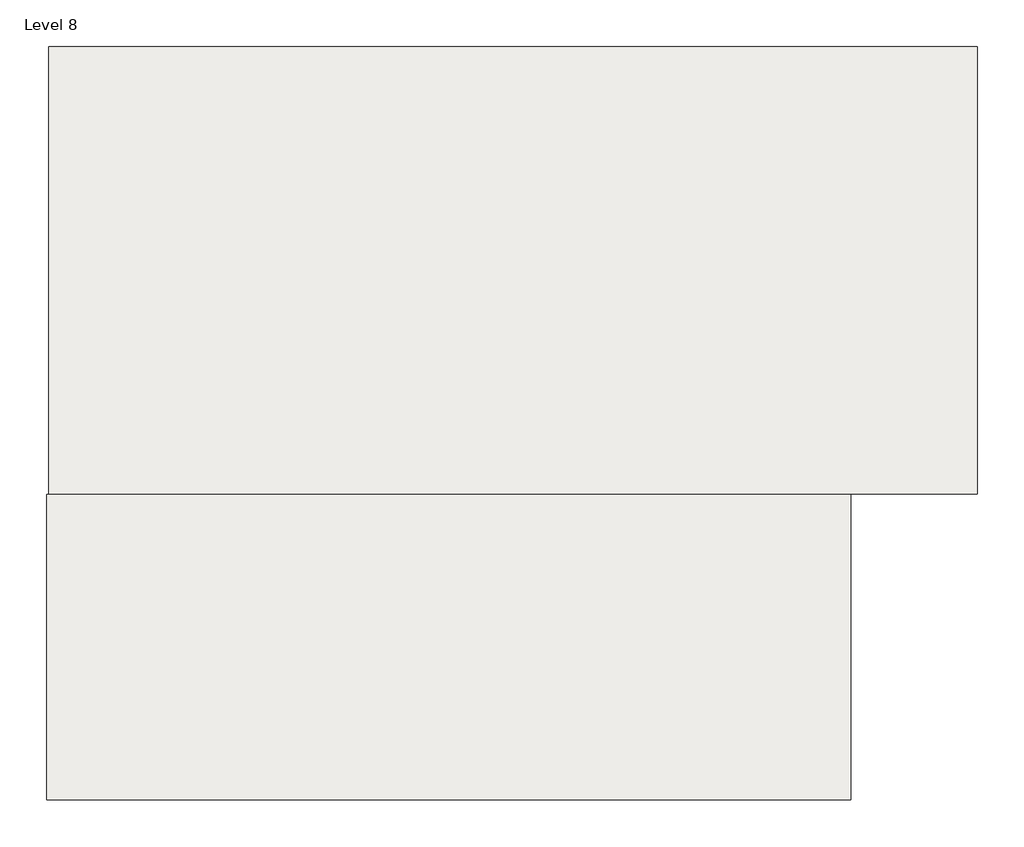
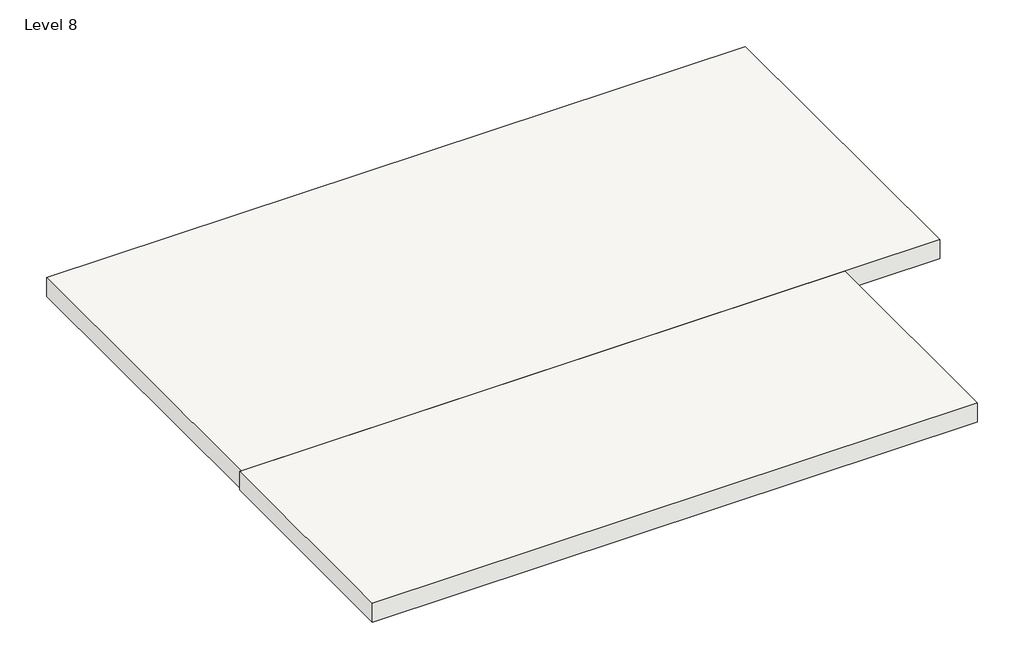
# One storey: 2 roofs.
"""IFC4 building model written with IfcOpenShell, lengths in millimetres."""

from ifc_helpers import new_model, si_unit, frame, origin, place, context, project, spatial, polyline, outline, extrude, element, save

model = new_model("IFC4")

# Units and contexts
model_context = context("Model", 3, world=origin())
ifc_project = project(units=[si_unit("LENGTHUNIT", "METRE", prefix="MILLI")], contexts=[model_context])

# Site, building, storey
site = spatial("IfcSite", under=ifc_project)
building = spatial("IfcBuilding", under=site)
storey = spatial("IfcBuildingStorey", under=building, Name="Level 8", Elevation=25603.2)

# Roofs
placement = place(None, origin())
element("IfcRoof", 1, ObjectType="Generic - 12\"", at=placement, inside=storey, context=model_context, shape_type="SweptSolid", body=[
    extrude(outline(polyline([(-14209.7864811, 5725.8297737), (-4862.5864811, 5725.8297737), (-4862.5864811, 2169.8297737), (-14209.7864811, 2169.8297737), (-14209.7864811, 5725.8297737)])), frame((0.0, 0.0, 25603.2), z_axis=(0.0, 0.0, 1.0), x_axis=(1.0, 0.0, 0.0)), (0.0, 0.0, 1.0), 304.8),
])
element("IfcRoof", 2, ObjectType="Generic - 12\"", at=placement, inside=storey, context=model_context, shape_type="SweptSolid", body=[
    extrude(outline(polyline([(-14184.3864811, 10932.8297737), (-3389.3864811, 10932.8297737), (-3389.3864811, 5726.6732783), (-14184.3864811, 5726.6732783), (-14184.3864811, 10932.8297737)])), frame((0.0, 0.0, 25603.2), z_axis=(0.0, 0.0, 1.0), x_axis=(1.0, 0.0, 0.0)), (0.0, 0.0, 1.0), 304.8),
])

save(model, "model.ifc")

# Revit data of these elements
# Type "Generic - 12\""
#   Assembly Code = "B1020"
#   Layers, outside or top first: 1' - 0" no material (function 1)
# Elements 1, 2 (IfcRoof, "Generic - 12\"")
#   built-in parameter 1001705 = 85 (stored number, unit not read)
#   built-in parameter 1001710 = 33615
#   Phase Created = New Construction
#   Materials on its faces: "Default Roof"
# Materials
#   "Default Roof": colour RGB 88 101 114, transparency 0
